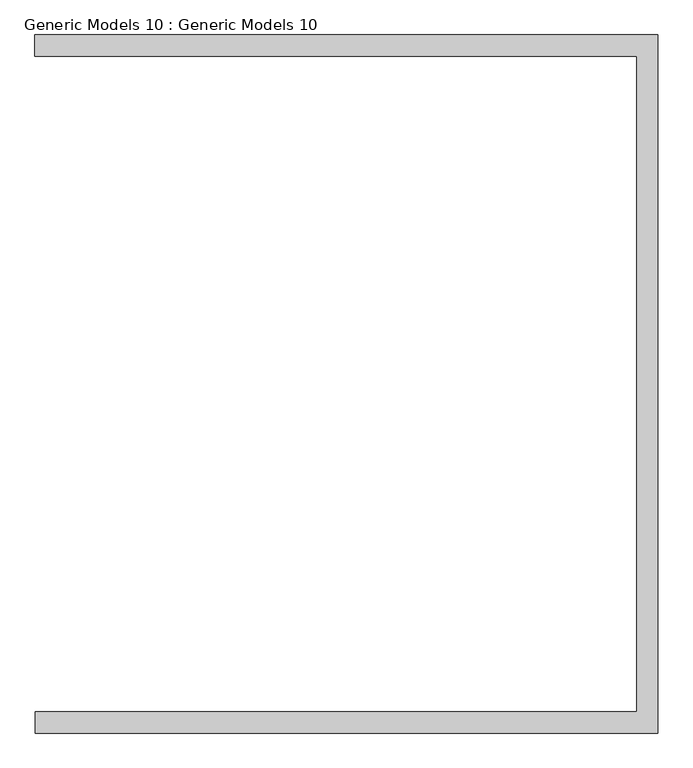
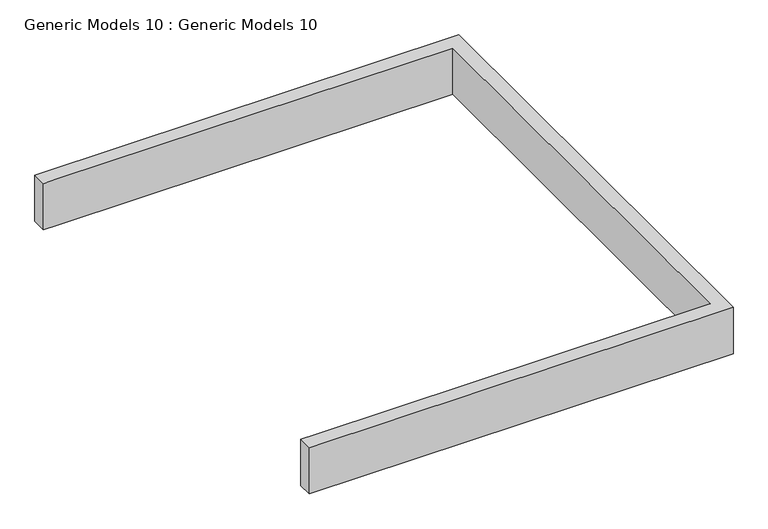
"""IFC4 building model written with IfcOpenShell, lengths in millimetres: proxy geometry, Generic Models 10 : Generic Models 10."""

from ifc_helpers import new_model, si_unit, origin, place, context, project, spatial, faceted_brep, source, transform, mapped, element, save


def generic_models_10_generic_models_10_cbb95902(model_context):
    return source(origin(), model_context, "Body", "Brep", [
        faceted_brep([(-21408.9206529, -16864.2026331, 1483.4369838), (-21408.9206529, -16864.2026331, -304.8), (-5890.1125638, -16864.2026331, -304.8), (-5890.1125638, -16864.2026331, 1483.4369838), (-6423.5125638, -16330.8026331, -304.8), (-20900.9206529, -16330.8026331, -304.8), (-21408.9206529, -16330.8026331, -304.8), (-21408.9206529, -16330.8026331, 1483.4369838), (-20900.9206529, -16330.8026331, 1483.4369838), (-6423.5125638, -16330.8026331, 1483.4369838), (-5890.1125638, 532.8888276, 1483.4369838), (-21416.2828462, 532.8888276, 1483.4369838), (-21416.2828462, -0.5111724, 1483.4369838), (-20900.9206529, -0.5111724, 1483.4369838), (-6423.5125638, -0.5111724, 1483.4369838), (-6423.5125638, -0.5111724, -304.8), (-20900.9206529, -0.5111724, -304.8), (-21416.2828462, -0.5111724, -304.8), (-21416.2828462, 532.8888276, -304.8), (-5890.1125638, 532.8888276, -304.8)], [[[0, 1, 2, 3]], [[4, 5, 6, 7, 8, 9]], [[9, 8, 7, 0, 3, 10, 11, 12, 13, 14]], [[1, 0, 7, 6]], [[6, 5, 4, 15, 16, 17, 18, 19, 2, 1]], [[10, 3, 2, 19]], [[15, 4, 9, 14]], [[19, 18, 11, 10]], [[12, 17, 16, 15, 14, 13]], [[11, 18, 17, 12]]]),
    ])


if __name__ == "__main__":
    model = new_model("IFC4")
    model_context = context("Model", 3, world=origin())
    ifc_project = project(units=[si_unit("LENGTHUNIT", "METRE", prefix="MILLI")], contexts=[model_context])
    site = spatial("IfcSite", under=ifc_project)
    building = spatial("IfcBuilding", under=site)
    placement = place(None, origin())
    generic_models_10_generic_models_10_shape = generic_models_10_generic_models_10_cbb95902(model_context)
    element("IfcBuildingElementProxy", 1, Name="Generic Models 10 : Generic Models 10", ObjectType="Generic Models 10 : Generic Models 10", at=placement, inside=building, context=model_context, shape_type="MappedRepresentation", body=[
        mapped(generic_models_10_generic_models_10_shape, transform((0.0, 0.0, 0.0), x_axis=(1.0, 0.0, 0.0), y_axis=(0.0, 1.0, 0.0), z_axis=(0.0, 0.0, 1.0))),
    ])
    save(model, "model.ifc")
